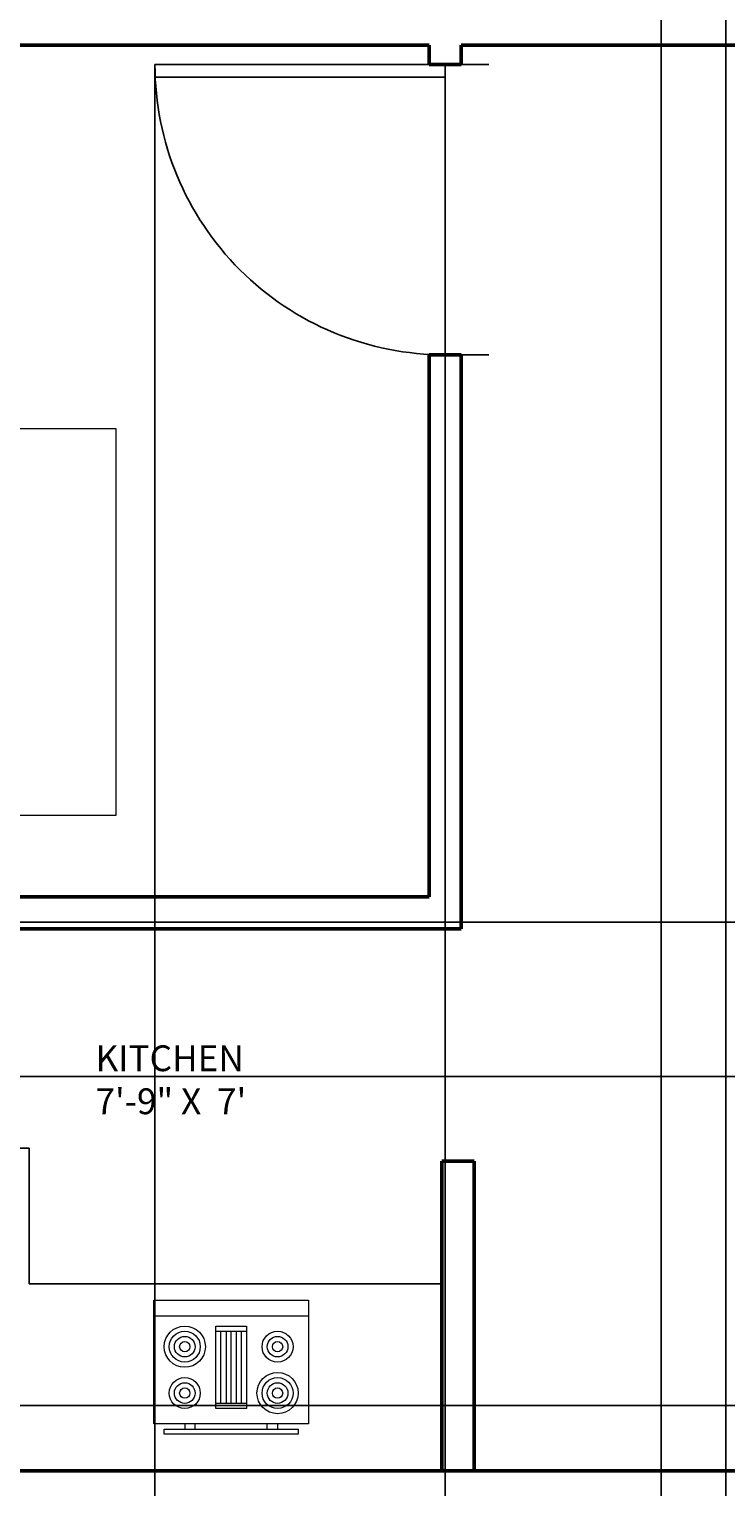
# Model space of a CAD drawing. Units: inches. Extents: x 3506 to 3958, y 1553 to 2506.
# Tile 10 of 16: x 3631 to 3739, y 2003 to 2229. Entities that reach past the tile are written whole.
import ezdxf

# ---------------------------------------------------------------- set-up
doc = ezdxf.new("R2010")
doc.units = ezdxf.units.IN
doc.header["$MEASUREMENT"] = 0
for name, color, linetype, lineweight in [('A-ANNO-DIMS', 2, 'Continuous', 18), ('A-AREA-IDEN', 7, 'Continuous', 18), ('A-FLOR-CASE', 7, 'Continuous', 25), ('A-WALL', 7, 'Continuous', 50), ('doors', 40, 'Continuous', 25), ('furniture', 120, 'Continuous', 18), ('kitchen', 181, 'Continuous', 18)]:
    doc.layers.add(name, color=color, linetype=linetype, lineweight=lineweight)
doc.layers.add('A-WALL-PATT', color=251, linetype='Continuous', lineweight=13, true_color=0x636466)
doc.styles.get("Standard").update_dxf_attribs({"font": 'arial.ttf'})
doc.dimstyles.get("Standard").update_dxf_attribs({"dimtxt": 1.18, "dimasz": 0.68, "dimexe": 0.18, "dimexo": 0.0625, "dimgap": 0.09, "dimtad": 0, "dimtih": 1, "dimtoh": 1, "dimdec": 1, "dimzin": 0, "dimdsep": 46, "dimlunit": 3, "dimtxsty": 'Standard', "dimcen": 0.09, "dimadec": 0, "dimazin": 0, "dimtfac": 1, "dimtdec": 1, "dimtofl": 0, "dimtmove": 0, "dimatfit": 3, "dimfxl": 1, "dimtolj": 1, "dimtzin": 0, "dimarcsym": 0})

# ---------------------------------------------------------------- blocks, each defined once
blk = doc.blocks.new('*U12')
for p, q in [((0, 0), (0, 6)), ((40, 0), (40, 6))]:
    blk.add_line(p, q)
blk.add_lwpolyline([(0, 0), (0, -40), (1.75, -40), (1.75, 0)], close=True)
blk.add_arc((0, 0), 40, 270, 0)
blk = doc.blocks.new('Bed - Queen')
for p, q in [((0, -80.00003), (0, 0)), ((0, 0), (59.99999, 0)), ((59.99999, 0), (59.99999, -80.00003)), ((7.99999, -1.2), (28.79998, -1.2)), ((7.99999, -14.4), (7.99999, -1.2)), ((28.79998, -1.2), (28.79998, -14.4)), ((31.19999, -1.2), (51.99999, -1.2)), ((31.19999, -14.4), (31.19999, -1.2)), ((51.99999, -1.2), (51.99999, -16.4)), ((0, -14.4), (44.8, -14.4)), ((59.99999, -29.6), (44.8, -14.4)), ((44.8, -14.4), (44.8, -29.6)), ((44.8, -16.8), (0, -16.8)), ((51.99999, -16.4), (46.79936, -16.4)), ((44.8, -29.6), (59.99999, -29.6)), ((59.99999, -80.00003), (0, -80.00003))]:
    blk.add_line(p, q)
blk = doc.blocks.new('Range-Oven - 30 in top')
for p, q in [((0, -3), (30, -3)), ((12, -6), (18, -6)), ((13, -20), (13, -6)), ((14, -6), (14, -20)), ((15, -20), (15, -6)), ((16, -6), (16, -20)), ((17, -20), (17, -6)), ((18, -20), (12, -20)), ((6, -24), (6, -25)), ((8, -25), (8, -24)), ((22, -25), (22, -24)), ((24, -24), (24, -25))]:
    blk.add_line(p, q)
for points in [[(0, -24), (0, 0), (30, 0), (30, -24)], [(12, -21), (12, -5), (18, -5), (18, -21)], [(2, -26), (2, -25), (28, -25), (28, -26)]]:
    blk.add_lwpolyline(points, close=True)
for centre, radius in [((6, -9), 4), ((6, -9), 3), ((6, -9), 2), ((6, -9), 1), ((24, -9), 3), ((24, -9), 2), ((24, -9), 1), ((24, -18), 4), ((6, -18), 3), ((6, -18), 2), ((24, -18), 3), ((24, -18), 2), ((6, -18), 1), ((24, -18), 1)]:
    blk.add_circle(centre, radius)
blk = doc.blocks.new('*D44')
at = {"layer": 'A-ANNO-DIMS', "color": 0, "lineweight": -2, "transparency": 16777216}
for p, q in [((3911.67, 2461.39), (3508.1, 2461.39)), ((3508.28, 2460.71), (3508.28, 2344.59)), ((3508.28, 2227.07), (3508.28, 2343.2)), ((3560.67, 2226.39), (3508.1, 2226.39))]:
    blk.add_line(p, q, dxfattribs=at)
at = {"layer": 'A-ANNO-DIMS', "color": 0, "transparency": 16777216}
for points in [[(3508.17, 2460.71), (3508.39, 2460.71), (3508.28, 2461.39)], [(3508.17, 2227.07), (3508.39, 2227.07), (3508.28, 2226.39)]]:
    blk.add_solid(points, dxfattribs=at)
at = {"layer": 'Defpoints', "color": 0, "transparency": 16777216}
for p in [(3508.28, 2461.39), (3911.73, 2461.39), (3560.73, 2226.39)]:
    blk.add_point(p, dxfattribs=at)
at = {"layer": 'A-ANNO-DIMS', "color": 0, "transparency": 16777216, "insert": (3508.28, 2343.89), "char_height": 1.18, "attachment_point": 5}
blk.add_mtext('\\A1;235', dxfattribs=at)
blk = doc.blocks.new('*D50')
at = {"layer": 'A-ANNO-DIMS', "color": 0, "lineweight": -2, "transparency": 16777216}
for p, q in [((3608.73, 1606.46), (3608.73, 2505.02)), ((3609.41, 2504.84), (3672.39, 2504.84)), ((3738.05, 2504.84), (3675.07, 2504.84)), ((3738.73, 1606.46), (3738.73, 2505.02))]:
    blk.add_line(p, q, dxfattribs=at)
at = {"layer": 'A-ANNO-DIMS', "color": 0, "transparency": 16777216}
for points in [[(3609.41, 2504.96), (3609.41, 2504.73), (3608.73, 2504.84)], [(3738.05, 2504.96), (3738.05, 2504.73), (3738.73, 2504.84)]]:
    blk.add_solid(points, dxfattribs=at)
at = {"layer": 'Defpoints', "color": 0, "transparency": 16777216}
for p in [(3738.73, 2504.84), (3608.73, 1606.39), (3738.73, 1606.39)]:
    blk.add_point(p, dxfattribs=at)
at = {"layer": 'A-ANNO-DIMS', "color": 0, "transparency": 16777216, "insert": (3673.73, 2504.84), "char_height": 1.18, "attachment_point": 5}
blk.add_mtext('\\A1;130', dxfattribs=at)
blk = doc.blocks.new('*D59')
at = {"layer": 'A-ANNO-DIMS', "color": 0, "lineweight": -2, "transparency": 16777216}
for p, q in [((3728.73, 1689.46), (3728.73, 2505.02)), ((3729.41, 2504.84), (3732.85, 2504.84)), ((3738.05, 2504.84), (3734.61, 2504.84)), ((3738.73, 1689.46), (3738.73, 2505.02))]:
    blk.add_line(p, q, dxfattribs=at)
at = {"layer": 'A-ANNO-DIMS', "color": 0, "transparency": 16777216}
for points in [[(3729.41, 2504.96), (3729.41, 2504.73), (3728.73, 2504.84)], [(3738.05, 2504.96), (3738.05, 2504.73), (3738.73, 2504.84)]]:
    blk.add_solid(points, dxfattribs=at)
at = {"layer": 'Defpoints', "color": 0, "transparency": 16777216}
for p in [(3738.73, 2504.84), (3728.73, 1689.39), (3738.73, 1689.39)]:
    blk.add_point(p, dxfattribs=at)
at = {"layer": 'A-ANNO-DIMS', "color": 0, "transparency": 16777216, "insert": (3733.73, 2504.84), "char_height": 1.18, "attachment_point": 5}
blk.add_mtext('\\A1;10', dxfattribs=at)
blk = doc.blocks.new('*D60')
at = {"layer": 'A-ANNO-DIMS', "color": 0, "lineweight": -2, "transparency": 16777216}
for p, q in [((3860.67, 2066.52), (3508.1, 2066.52)), ((3508.28, 2065.84), (3508.28, 2041.7)), ((3508.28, 2016.17), (3508.28, 2040.31)), ((3860.67, 2015.49), (3508.1, 2015.49))]:
    blk.add_line(p, q, dxfattribs=at)
at = {"layer": 'A-ANNO-DIMS', "color": 0, "transparency": 16777216}
for points in [[(3508.17, 2065.84), (3508.39, 2065.84), (3508.28, 2066.52)], [(3508.17, 2016.17), (3508.39, 2016.17), (3508.28, 2015.49)]]:
    blk.add_solid(points, dxfattribs=at)
at = {"layer": 'Defpoints', "color": 0, "transparency": 16777216}
for p in [(3860.73, 2066.52), (3508.28, 2015.49), (3860.73, 2015.49)]:
    blk.add_point(p, dxfattribs=at)
at = {"layer": 'A-ANNO-DIMS', "color": 0, "transparency": 16777216, "insert": (3508.28, 2041), "char_height": 1.18, "attachment_point": 5}
blk.add_mtext('\\A1;51.03', dxfattribs=at)
blk = doc.blocks.new('*D61')
at = {"layer": 'A-ANNO-DIMS', "color": 0, "lineweight": -2, "transparency": 16777216}
for p, q in [((3860.67, 2090.43), (3508.1, 2090.43)), ((3508.28, 2089.75), (3508.28, 2079.17)), ((3508.28, 2067.2), (3508.28, 2077.78)), ((3860.67, 2066.52), (3508.1, 2066.52))]:
    blk.add_line(p, q, dxfattribs=at)
at = {"layer": 'A-ANNO-DIMS', "color": 0, "transparency": 16777216}
for points in [[(3508.17, 2089.75), (3508.39, 2089.75), (3508.28, 2090.43)], [(3508.17, 2067.2), (3508.39, 2067.2), (3508.28, 2066.52)]]:
    blk.add_solid(points, dxfattribs=at)
at = {"layer": 'Defpoints', "color": 0, "transparency": 16777216}
for p in [(3860.73, 2090.43), (3508.28, 2066.52), (3860.73, 2066.52)]:
    blk.add_point(p, dxfattribs=at)
at = {"layer": 'A-ANNO-DIMS', "color": 0, "transparency": 16777216, "insert": (3508.28, 2078.48), "char_height": 1.18, "attachment_point": 5}
blk.add_mtext('\\A1;23.92', dxfattribs=at)
blk = doc.blocks.new('*D66')
at = {"layer": 'A-ANNO-DIMS', "color": 0, "lineweight": -2, "transparency": 16777216}
for p, q in [((3650.23, 2221.36), (3650.23, 1553.76)), ((3695.23, 2221.36), (3695.23, 1553.76)), ((3650.91, 1553.94), (3671.77, 1553.94)), ((3694.55, 1553.94), (3673.69, 1553.94))]:
    blk.add_line(p, q, dxfattribs=at)
at = {"layer": 'A-ANNO-DIMS', "color": 0, "transparency": 16777216}
for points in [[(3650.91, 1554.06), (3650.91, 1553.83), (3650.23, 1553.94)], [(3694.55, 1554.06), (3694.55, 1553.83), (3695.23, 1553.94)]]:
    blk.add_solid(points, dxfattribs=at)
at = {"layer": 'Defpoints', "color": 0, "transparency": 16777216}
for p in [(3650.23, 2221.43), (3695.23, 2221.43), (3695.23, 1553.94)]:
    blk.add_point(p, dxfattribs=at)
at = {"layer": 'A-ANNO-DIMS', "color": 0, "transparency": 16777216, "insert": (3672.73, 1553.94), "char_height": 1.18, "attachment_point": 5}
blk.add_mtext('\\A1;45', dxfattribs=at)

msp = doc.modelspace()

# ---------------------------------------------------------------- hatches: boundary and pattern name
at = {"layer": 'A-WALL-PATT'}
h = msp.add_hatch(dxfattribs=at)
h.set_pattern_fill('ANSI31', color=256)
h.paths.add_polyline_path([(3911.7302, 2461.3942), (3551.7302, 2461.3942), (3551.7302, 2152.516), (3560.7302, 2152.516), (3560.7302, 2116.516), (3551.7302, 2116.516), (3551.7302, 1920.5711), (3556.2302, 1920.5711), (3560.7302, 1920.5711), (3560.7302, 2000.3942), (3692.7302, 2000.3942), (3692.7302, 1997.3942), (3697.7302, 1997.3942), (3697.7302, 2000.3942), (3771.7302, 2000.3942), (3771.7302, 1997.3942), (3776.7302, 1997.3942), (3776.7302, 1997.7206), (3778.5802, 1997.7206), (3807.5802, 1997.7206), (3807.5802, 1996.4519), (3778.5802, 1996.4519), (3778.5802, 1997.7206), (3776.7302, 1997.7206), (3776.7302, 1997.3942), (3771.7302, 1997.3942), (3771.7302, 2000.3942), (3697.7302, 2000.3942), (3697.7302, 1997.3942), (3692.7302, 1997.3942), (3689.8302, 1997.3942), (3689.8302, 1995.8192), (3653.8302, 1995.8192), (3653.8302, 1997.3942), (3689.8302, 1997.3942), (3692.7302, 1997.3942), (3692.7302, 2000.3942), (3560.7302, 2000.3942), (3560.7302, 1920.5711), (3551.7302, 1920.5711), (3551.7302, 1884.5711), (3551.7302, 1597.3942), (3911.7302, 1597.3942)], flags=17)
h.paths.add_polyline_path([(3596.7302, 2005.3942), (3596.7302, 2057.3035, -0.38730371), (3569.1778, 2085), (3569.15, 2085), (3569.15, 2086.2688), (3598.15, 2086.2688), (3598.15, 2085), (3569.1778, 2085, 0.38730371), (3596.7302, 2057.3035), (3596.7302, 2057.3942), (3601.7302, 2057.3942), (3601.7302, 2055.3942), (3630.7302, 2055.3942), (3630.7302, 2034.3942), (3694.7302, 2034.3942), (3694.7302, 2053.3942), (3699.7302, 2053.3942), (3699.7302, 2005.3942), (3860.7302, 2005.3942), (3860.7302, 2173.3942), (3771.7302, 2173.3942), (3771.7302, 2194.3942), (3776.7302, 2194.3942), (3776.7302, 2178.3942), (3860.7302, 2178.3942), (3860.7302, 2231.3942), (3601.7302, 2231.3942), (3601.7302, 2241.426), (3596.7302, 2241.426), (3596.7302, 2231.3942), (3560.7302, 2231.3942), (3560.7302, 2315.3942), (3596.7302, 2315.3942), (3596.7302, 2312.3942), (3601.7302, 2312.3942), (3601.7302, 2315.3942), (3697.7302, 2315.3942), (3697.7302, 2413.3942), (3692.7302, 2413.3942), (3692.7302, 2320.3942), (3560.7302, 2320.3942), (3560.7302, 2452.3942), (3692.7302, 2452.3942), (3692.7302, 2449.3942), (3697.7302, 2449.3942), (3697.7302, 2452.3942), (3771.7302, 2452.3942), (3771.7302, 2449.3942), (3776.7302, 2449.3942), (3776.7302, 2452.3942), (3860.7302, 2452.3942), (3860.7302, 2437.2075), (3865.2302, 2437.2075), (3865.2302, 2413.2075), (3860.7302, 2413.2075), (3860.7302, 2367.6976), (3865.2302, 2367.6976), (3869.7302, 2367.6976), (3869.7302, 2319.6976), (3860.7302, 2319.6976), (3860.7302, 2211.6248), (3869.7302, 2211.6248), (3869.7302, 2187.6248), (3860.7302, 2187.6248), (3860.7302, 2138.4346), (3865.2302, 2138.4346), (3869.7302, 2138.4346), (3869.7302, 2090.4346), (3860.7302, 2090.4346), (3860.7302, 1985.8449), (3869.7302, 1985.8449), (3869.7302, 1961.8449), (3860.7302, 1961.8449), (3860.7302, 1897.0756), (3865.2302, 1897.0756), (3869.7302, 1897.0756), (3869.7302, 1849.0756), (3860.7302, 1849.0756), (3860.7302, 1847.8112), (3860.7302, 1779.3942), (3596.7302, 1779.3942), (3596.7302, 1831.3942), (3601.7302, 1831.3942), (3601.7302, 1828.3942), (3630.7302, 1828.3942), (3630.7302, 1808.3942), (3691.7302, 1808.3942), (3691.7302, 1815.3942), (3696.7302, 1815.3942), (3696.7302, 1779.3942), (3860.7302, 1779.3942), (3860.7302, 1947.3942), (3771.7302, 1947.3942), (3771.7302, 1968.3942), (3776.7302, 1968.3942), (3776.7302, 1952.3942), (3860.7302, 1952.3942), (3860.7302, 2005.3942)], flags=0)
h.paths.add_polyline_path([(3596.7302, 2038.8546), (3601.7302, 2038.8546), (3601.7302, 2014.8546), (3596.7302, 2014.8546)], flags=0)
h.paths.add_polyline_path([(3564.1688, 2107), (3564.1688, 2167), (3644.1688, 2167), (3644.1688, 2107)], flags=0)
h.paths.add_polyline_path([(3607.0972, 2052.0208), (3620.8472, 2052.0208, -0.41421356), (3621.9931, 2050.875), (3621.9931, 2025.6667, -0.41421356), (3620.8472, 2024.5208), (3607.0972, 2024.5208, -0.41421356), (3605.9514, 2025.6667), (3605.9514, 2050.875, -0.41421356)], flags=0)
h.paths.add_polyline_path([(3578.5688, 2115), (3565.3688, 2115), (3565.3688, 2135.8), (3578.5688, 2135.8), (3578.5688, 2138.2), (3565.3688, 2138.2), (3565.3688, 2159), (3580.5688, 2159), (3580.5688, 2153.8), (3593.7688, 2167), (3593.7688, 2151.8), (3578.5688, 2151.8)], flags=0)
h.paths.add_polyline_path([(3610.9167, 2050.875), (3620.0833, 2050.875, -0.41421356), (3620.8472, 2050.1111), (3620.8472, 2039.6076, -0.41421356), (3620.0833, 2038.8438), (3610.9167, 2038.8438, -0.41421356), (3610.1528, 2039.6076), (3610.1528, 2050.1111, -0.41421356)], flags=0)
h.paths.add_polyline_path([(3610.9167, 2037.6979), (3620.0833, 2037.6979, -0.41421356), (3620.8472, 2036.934), (3620.8472, 2026.4306, -0.41421356), (3620.0833, 2025.6667), (3610.9167, 2025.6667, -0.41421356), (3610.1528, 2026.4306), (3610.1528, 2036.934, -0.41421356)], flags=0)
h.paths.add_polyline_path([(3616.2639, 2044.7639, -1), (3614.7361, 2044.7639, -1)], flags=0)
h.paths.add_polyline_path([(3615.8819, 2044.7639, -1), (3615.1181, 2044.7639, -1)], flags=0)
h.paths.add_polyline_path([(3616.2639, 2031.7778, -1), (3614.7361, 2031.7778, -1)], flags=0)
h.paths.add_polyline_path([(3615.8819, 2031.7778, -1), (3615.1181, 2031.7778, -1)], flags=0)
h.paths.add_polyline_path([(3609.7539, 2021.7868), (3626.9586, 2021.7868), (3626.9586, 2008.8833), (3609.7539, 2008.8833)], flags=0)
h.paths.add_polyline_path([(3610.4708, 2021.07), (3621.2237, 2021.07), (3621.2237, 2009.6002), (3610.4708, 2009.6002)], flags=0)
h.paths.add_polyline_path([(3611.5461, 2019.9947), (3620.1484, 2019.9947), (3620.1484, 2010.6755), (3611.5461, 2010.6755)], flags=0)
h.paths.add_polyline_path([(3621.9405, 2021.07), (3626.2417, 2021.07), (3626.2417, 2009.6002), (3621.9405, 2009.6002)], flags=0)
h.paths.add_polyline_path([(3622.6574, 2020.3531), (3625.5248, 2020.3531), (3625.5248, 2017.4857), (3622.6574, 2017.4857)], flags=0)
h.paths.add_polyline_path([(3622.6574, 2016.7688), (3625.5248, 2016.7688), (3625.5248, 2010.317), (3622.6574, 2010.317)], flags=0)
h.paths.add_polyline_path([(3624.808, 2016.0519), (3624.808, 2013.9013), (3624.0911, 2013.9013), (3624.0911, 2013.1845), (3623.3743, 2013.1845), (3623.3743, 2013.9013), (3623.3743, 2016.0519)], flags=0)
h.paths.add_polyline_path([(3623.0158, 2012.8261), (3625.1664, 2012.8261), (3625.1664, 2012.1092), (3623.0158, 2012.1092)], flags=0)
h.paths.add_polyline_path([(3623.0158, 2011.7508), (3625.1664, 2011.7508), (3625.1664, 2011.0339), (3623.0158, 2011.0339)], flags=0)
h.paths.add_polyline_path([(3650.0591, 2031.8202), (3674.0368, 2031.8202), (3674.0368, 2012.638), (3669.2413, 2012.638), (3669.2413, 2011.8388), (3672.4383, 2011.8388), (3672.4383, 2011.0395), (3651.6576, 2011.0395), (3651.6576, 2011.8388), (3654.8546, 2011.8388), (3654.8546, 2012.638), (3650.0591, 2012.638)], flags=0)
h.paths.add_polyline_path([(3658.0517, 2024.6269, -1), (3651.6576, 2024.6269, -1)], flags=0)
h.paths.add_polyline_path([(3657.2524, 2024.6269, -1), (3652.4569, 2024.6269, -1)], flags=0)
h.paths.add_polyline_path([(3656.4532, 2024.6269, -1), (3653.2561, 2024.6269, -1)], flags=0)
h.paths.add_polyline_path([(3655.6539, 2024.6269, -1), (3654.0554, 2024.6269, -1)], flags=0)
h.paths.add_polyline_path([(3657.2524, 2017.4336, -1), (3652.4569, 2017.4336, -1)], flags=0)
h.paths.add_polyline_path([(3656.4532, 2017.4336, -1), (3653.2561, 2017.4336, -1)], flags=0)
h.paths.add_polyline_path([(3655.6539, 2017.4336, -1), (3654.0554, 2017.4336, -1)], flags=0)
h.paths.add_polyline_path([(3659.6502, 2027.8239), (3664.4457, 2027.8239), (3664.4457, 2015.0358), (3659.6502, 2015.0358)], flags=0)
h.paths.add_polyline_path([(3663.6465, 2027.0247), (3663.6465, 2015.8351), (3660.4494, 2015.8351), (3660.4494, 2027.0247)], flags=0)
h.paths.add_polyline_path([(3562.6688, 1945.5), (3642.6688, 1945.5), (3642.6688, 1885.5), (3562.6688, 1885.5)], flags=0)
h.paths.add_polyline_path([(3671.6391, 2024.6269, -1), (3666.8435, 2024.6269, -1)], flags=0)
h.paths.add_polyline_path([(3670.8398, 2024.6269, -1), (3667.6428, 2024.6269, -1)], flags=0)
h.paths.add_polyline_path([(3672.4383, 2017.4336, -1), (3666.0443, 2017.4336, -1)], flags=0)
h.paths.add_polyline_path([(3670.0405, 2024.6269, -1), (3668.442, 2024.6269, -1)], flags=0)
h.paths.add_polyline_path([(3671.6391, 2017.4336, -1), (3666.8435, 2017.4336, -1)], flags=0)
h.paths.add_polyline_path([(3670.8398, 2017.4336, -1), (3667.6428, 2017.4336, -1)], flags=0)
h.paths.add_polyline_path([(3592.2688, 1945.5), (3592.2688, 1930.3), (3577.0688, 1930.3), (3577.0688, 1893.5), (3563.8688, 1893.5), (3563.8688, 1914.3), (3577.0688, 1914.3), (3577.0688, 1916.7), (3563.8688, 1916.7), (3563.8688, 1937.5), (3579.0688, 1937.5), (3579.0688, 1932.3)], flags=0)
h.paths.add_polyline_path([(3670.0405, 2017.4336, -1), (3668.442, 2017.4336, -1)], flags=0)
h.paths.add_polyline_path([(3596.7302, 2283.3942), (3601.7302, 2283.3942), (3601.7302, 2265.426), (3599.2302, 2265.426), (3599.2302, 2241.426), (3596.7302, 2241.426), (3596.7302, 2265.426)], flags=0)
h.paths.add_polyline_path([(3596.7302, 1810.7006), (3601.7302, 1810.7006), (3601.7302, 1786.7006), (3596.7302, 1786.7006)], flags=0)
h.paths.add_polyline_path([(3560.7302, 1770.3942), (3738.7302, 1770.3942), (3738.7302, 1746.3942), (3738.7302, 1722.3942), (3748.7302, 1722.3942), (3748.7302, 1674.3942), (3560.7302, 1674.3942)], flags=0)
h.paths.add_polyline_path([(3728.7302, 1746.3942), (3728.7302, 1756.0642), (3738.7302, 1746.3942), (3728.7302, 1738.1582), (3728.7302, 1698.3942), (3591.2519, 1698.3942), (3591.2519, 1746.3942)], flags=0)
h.paths.add_polyline_path([(3771.7302, 2399.3942), (3771.7302, 2420.3942), (3776.7302, 2420.3942), (3776.7302, 2404.3942), (3776.7302, 2399.3942)], flags=0)
h.paths.add_polyline_path([(3911.7302, 2461.3942), (3551.7302, 2461.3942), (3551.7302, 2152.516), (3560.7302, 2152.516), (3560.7302, 2116.516), (3551.7302, 2116.516), (3551.7302, 1920.5711), (3560.7302, 1920.5711), (3560.7302, 2000.3942), (3692.7302, 2000.3942), (3692.7302, 1997.3942), (3697.7302, 1997.3942), (3697.7302, 2000.3942), (3771.7302, 2000.3942), (3771.7302, 1997.3942), (3776.7302, 1997.3942), (3776.7302, 1997.7206), (3778.5802, 1997.7206), (3807.5802, 1997.7206), (3807.5802, 1996.4519), (3778.5802, 1996.4519), (3778.5802, 1997.7206), (3776.7302, 1997.7206), (3776.7302, 1997.3942), (3771.7302, 1997.3942), (3771.7302, 2000.3942), (3697.7302, 2000.3942), (3697.7302, 1997.3942), (3692.7302, 1997.3942), (3689.8302, 1997.3942), (3689.8302, 1995.8192), (3653.8302, 1995.8192), (3653.8302, 1997.3942), (3689.8302, 1997.3942), (3692.7302, 1997.3942), (3692.7302, 2000.3942), (3560.7302, 2000.3942), (3560.7302, 1920.5711), (3551.7302, 1920.5711), (3551.7302, 1597.3942), (3911.7302, 1597.3942)], flags=17)

# ---------------------------------------------------------------- linework, layer by layer
at = {"layer": 'A-FLOR-CASE'}
for p, q in [((3601.7302, 2055.3942), (3630.7302, 2055.3942)), ((3630.7302, 2034.3942), (3630.7302, 2055.3942)), ((3630.7302, 2034.3942), (3694.7302, 2034.3942))]:
    msp.add_line(p, q, dxfattribs=at)
at = {"layer": 'A-WALL'}
for p, q in [((3560.7302, 2226.3942), (3692.7302, 2226.3942)), ((3692.7302, 2226.3942), (3692.7302, 2223.3942)), ((3692.7302, 2223.3942), (3692.7302, 2226.3942)), ((3697.7302, 2226.3942), (3771.362, 2226.3942)), ((3697.7302, 2223.3942), (3697.7302, 2226.3942)), ((3692.7302, 2223.3942), (3697.7302, 2223.3942)), ((3692.7302, 2094.3942), (3692.7302, 2178.3942)), ((3692.7302, 2178.3942), (3697.7302, 2178.3942)), ((3697.7302, 2089.3942), (3697.7302, 2178.3942)), ((3560.7302, 2094.3942), (3692.7302, 2094.3942)), ((3601.7302, 2089.3942), (3697.7302, 2089.3942)), ((3694.7302, 2053.3942), (3699.7302, 2053.3942)), ((3694.7302, 2005.3942), (3694.7302, 2053.3942)), ((3699.7302, 2005.3942), (3699.7302, 2053.3942)), ((3560.7302, 2005.3942), (3860.7302, 2005.3942))]:
    msp.add_line(p, q, dxfattribs=at)

# ---------------------------------------------------------------- block references
at = {"layer": 'doors', "xscale": 1.124999999999988, "yscale": 1.124999999999988, "zscale": 1.124999999999988, "rotation": 270}
msp.add_blockref('*U12', (3695.2302, 2223.3942), dxfattribs=at)
at = {"layer": 'furniture', "rotation": 90}
msp.add_blockref('Bed - Queen', (3564.1688, 2107), dxfattribs=at)
at = {"layer": 'kitchen', "xscale": 0.7992583991282335, "yscale": 0.7992583991282335, "zscale": 0.7992583991282335}
msp.add_blockref('Range-Oven - 30 in top', (3650.0591, 2031.8202), dxfattribs=at)

# ---------------------------------------------------------------- texts
at = {"layer": 'A-AREA-IDEN', "insert": (3641.0073, 2071.3399), "char_height": 4, "attachment_point": 1}
msp.add_mtext_dynamic_manual_height_columns('KITCHEN\\P7\'-9" X  7\'', width=34.025371, gutter_width=1, heights=[0], dxfattribs=at)

# ---------------------------------------------------------------- dimensions: what is measured, and where the dimension line sits
at = {"layer": 'A-ANNO-DIMS'}
for base, p1, p2, picture, middle in [((3738.7302, 2504.8442), (3608.7302, 1606.3942), (3738.7302, 1606.3942), '*D50', (3673.7302, 2504.8442)), ((3738.7302, 2504.8442), (3728.7302, 1689.3942), (3738.7302, 1689.3942), '*D59', (3733.7302, 2504.8442)), ((3695.2302, 1553.9442), (3650.2302, 2221.4254), (3695.2302, 2221.4254), '*D66', (3672.7302, 1553.9442))]:
    dim = msp.add_linear_dim(base=base, p1=p1, p2=p2, dimstyle='Standard', override={"dimdec": 0, "dimlfac": 1, "dimrnd": 0, "dimzin": 0, "dimdsep": 46, "dimlunit": 2}, dxfattribs=at)
    dim.commit()
    dim.dimension.update_dxf_attribs({"geometry": picture, "text_midpoint": middle})
for base, p1, p2, override, picture, middle in [((3508.2802, 2461.3942), (3560.7302, 2226.3942), (3911.7302, 2461.3942), {"dimdec": 0, "dimlfac": 1, "dimrnd": 0, "dimzin": 0, "dimdsep": 46, "dimlunit": 2}, '*D44', (3508.2802, 2343.8942)), ((3508.2802, 2066.516), (3860.7302, 2090.4346), (3860.7302, 2066.516), {"dimdec": 2, "dimlfac": 1, "dimrnd": 0, "dimzin": 0, "dimdsep": 46, "dimlunit": 2}, '*D61', (3508.2802, 2078.4753)), ((3508.2802, 2015.4906), (3860.7302, 2066.516), (3860.7302, 2015.4906), {"dimdec": 2, "dimlfac": 1, "dimrnd": 0, "dimzin": 0, "dimdsep": 46, "dimlunit": 2}, '*D60', (3508.2802, 2041.0033))]:
    dim = msp.add_linear_dim(base=base, p1=p1, p2=p2, angle=90, dimstyle='Standard', override=override, dxfattribs=at)
    dim.commit()
    dim.dimension.update_dxf_attribs({"geometry": picture, "text_midpoint": middle})

doc.saveas('drawing.dxf')
